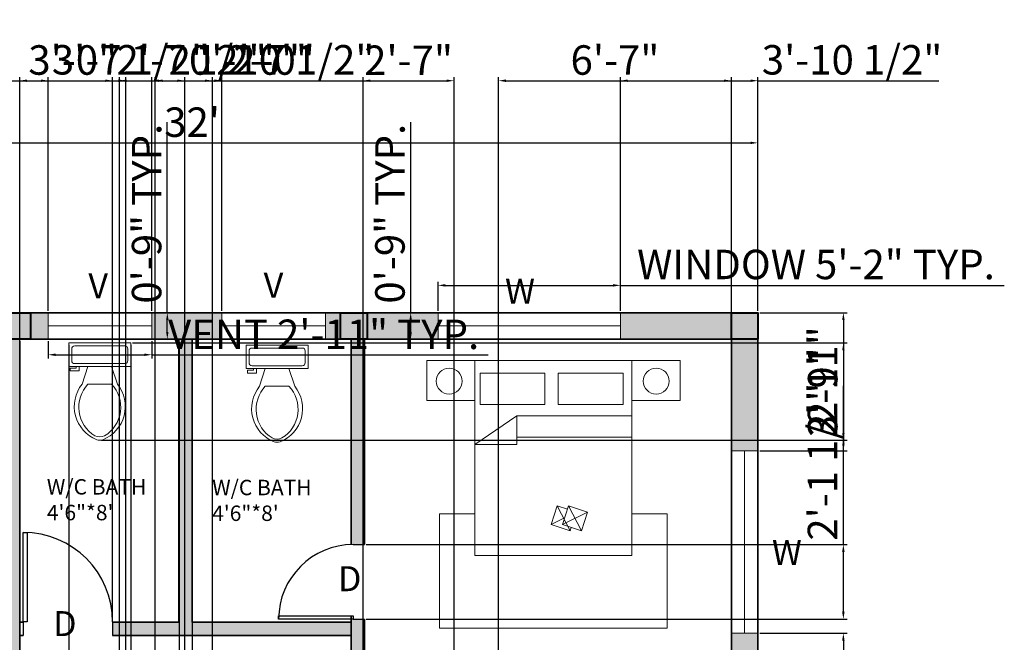
# Model space of a CAD drawing. Units: inches. Extents: x 1801 to 2333, y 2020 to 2714.
# Tile 4 of 4: x 1999 to 2333, y 2502 to 2714. Entities that reach past the tile are written whole.
import ezdxf

# ---------------------------------------------------------------- set-up
doc = ezdxf.new("R2010")
doc.units = ezdxf.units.IN
for name, color, linetype, lineweight in [('A-ANNO-DIMS', 2, 'Continuous', 18), ('A-ANNO-TEXT', 200, 'Continuous', 18), ('A-AREA-IDEN', 200, 'Continuous', 25), ('A-COLS', 7, 'Continuous', 40), ('A-COLS-PATT', 250, 'Continuous', 13), ('A-DOOR', 4, 'Continuous', 25), ('A-FLOR-FIXT', 9, 'Continuous', 18), ('A-FURN', 8, 'Continuous', 18), ('A-WALL-PATT', 252, 'Continuous', 13), ('WALL', 150, 'Continuous', 35), ('WINDOW', 130, 'Continuous', 18)]:
    doc.layers.add(name, color=color, linetype=linetype, lineweight=lineweight)
doc.styles.get("Standard").update_dxf_attribs({"font": 'arial.ttf'})
doc.dimstyles.new('ISO-25', dxfattribs={"dimtxt": 10, "dimasz": 2.5, "dimexe": 1.25, "dimexo": 0.625, "dimtad": 1, "dimdec": 0, "dimlunit": 4, "dimtxsty": 'Standard', "dimcen": 2.5, "dimadec": 0, "dimazin": 0, "dimtfac": 1, "dimtdec": 0, "dimtmove": 0, "dimatfit": 3, "dimfxl": 1, "dimarcsym": 0})

# ---------------------------------------------------------------- blocks, each defined once
blk = doc.blocks.new('*U2')
for p, q in [((0, 0), (0, -6)), ((40, 0), (40, -6))]:
    blk.add_line(p, q)
blk.add_lwpolyline([(0, 0), (0, 40), (1.75, 40), (1.75, 0)], close=True)
blk.add_arc((0, 0), 40, 0, 90)
blk = doc.blocks.new('*U4')
for p, q in [((9.5, -6), (9.5, -2)), ((-10, -8.5), (-8, -8.5)), ((-10, -9.5), (-10, -8.5)), ((-7, -9.5), (-10, -9.5)), ((-8, -8.5), (-8, -8)), ((-7, -8), (-7, -9.5)), ((-4, -8), (-6, -14)), ((4, -8), (6, -14)), ((4, -14), (-4, -14))]:
    blk.add_line(p, q)
blk.add_lwpolyline([(10.5, -8), (10.5, 0), (-10.5, 0), (-10.5, -8)], close=True)
for points in [[(-9.5, -2), (-9.5, -6)], [(8.5, -1), (-8.5, -1)], [(-8.5, -7), (8.5, -7)]]:
    blk.add_lwpolyline(points)
for centre, radius, start, end in [((-8.62, -1.88), 0.884, 81.8699, 188.1301), ((8.62, -1.88), 0.884, 351.8699, 98.1301), ((-8.62, -6.12), 0.884, 171.8699, 278.1301), ((8.62, -6.12), 0.884, 261.8699, 8.1301), ((3.52, -21.58), 12.17, 141.4691, 247.9714), ((4.2, -21.82), 11.33, 136.3677, 238.9468), ((-3.52, -21.58), 12.17, 292.0284, 38.5307), ((-4.2, -21.82), 11.33, 301.053, 43.6321), ((0, -27.88), 4, 245.7318, 294.2682), ((0, -29), 4, 254.8605, 285.1395)]:
    blk.add_arc(centre, radius, start, end)
blk = doc.blocks.new('*D7')
at = {"layer": 'A-ANNO-DIMS', "color": 0, "lineweight": -2, "transparency": 16777216}
for p, q in [((1865.69, 2614.97), (1865.69, 2673.24)), ((2249.69, 2614.97), (2249.69, 2673.24)), ((1868.19, 2671.99), (2247.19, 2671.99))]:
    blk.add_line(p, q, dxfattribs=at)
at = {"layer": 'A-ANNO-DIMS', "color": 0, "transparency": 16777216}
for points in [[(1868.19, 2672.4), (1868.19, 2671.57), (1865.69, 2671.99)], [(2247.19, 2672.4), (2247.19, 2671.57), (2249.69, 2671.99)]]:
    blk.add_solid(points, dxfattribs=at)
at = {"layer": 'Defpoints', "color": 0, "transparency": 16777216}
for p in [(2249.69, 2671.99), (1865.69, 2614.35), (2249.69, 2614.35)]:
    blk.add_point(p, dxfattribs=at)
at = {"layer": 'A-ANNO-DIMS', "color": 0, "transparency": 16777216, "insert": (2057.69, 2677.72), "char_height": 10, "attachment_point": 5}
blk.add_mtext("32'", dxfattribs=at)
blk = doc.blocks.new('BED-DOUBLE-WITH-NIGHTSTANDS')
for p, q in [((30.54, 72.05), (16.34, 62.37)), ((69.61, 72.05), (30.54, 72.05)), ((30.54, 62.37), (30.54, 72.05)), ((30.54, 64.89), (69.61, 64.89)), ((16.34, 62.37), (30.54, 62.37)), ((44.26, 41.5), (48.62, 33.08)), ((48.1, 41.5), (52.46, 33.08)), ((16.34, 38.79), (4.34, 38.79)), ((4.34, 38.79), (4.34, 0)), ((42.19, 35.19), (46.77, 37.46)), ((46.03, 35.19), (54.53, 39.39)), ((69.61, 38.79), (81.61, 38.79)), ((81.61, 38.79), (81.61, 0)), ((4.34, 0), (81.61, 0))]:
    blk.add_line(p, q)
for points in [[(0, 90.88), (16.34, 90.88), (16.34, 77.31), (0, 77.31)], [(16.34, 90.88), (69.61, 90.88), (69.61, 24.72), (16.34, 24.72)], [(69.61, 90.88), (85.96, 90.88), (85.96, 77.31), (69.61, 77.31)], [(18.06, 86.51), (40.1, 86.51), (40.1, 75.9), (18.06, 75.9)], [(44.61, 86.51), (66.65, 86.51), (66.65, 75.9), (44.61, 75.9)], [(46.03, 35.19), (48.1, 41.5), (54.53, 39.39), (52.46, 33.08)]]:
    blk.add_lwpolyline(points, close=True)
blk.add_lwpolyline([(48.99, 34.22), (48.62, 33.08), (42.19, 35.19), (44.26, 41.5), (47.73, 40.36)])
for centre in [(7.61, 83.86), (77.85, 83.86)]:
    blk.add_circle(centre, 4.4)
blk = doc.blocks.new('WIN-STANDARD')
blk.add_line((0, 4.5), (61.87, 4.5))
blk.add_lwpolyline([(0, 9), (61.87, 9), (61.87, 0), (0, 0)], close=True)
blk = doc.blocks.new('VENT-BATH')
blk.add_line((0, 4.5), (35.14, 4.5))
blk.add_lwpolyline([(0, 9), (35.14, 9), (35.14, 0), (0, 0)], close=True)
blk = doc.blocks.new('COLUMN-9X9')
blk.add_lwpolyline([(0, 9), (9, 9), (9, 0), (0, 0)], close=True)
blk = doc.blocks.new('*D18')
at = {"layer": 'A-ANNO-DIMS', "color": 0, "lineweight": -2, "transparency": 16777216}
for p, q in [((2141.14, 2614.97), (2141.14, 2624.88)), ((2143.64, 2623.63), (2200.51, 2623.63)), ((2203.01, 2614.97), (2203.01, 2624.88)), ((2203.01, 2623.63), (2333.3, 2623.63))]:
    blk.add_line(p, q, dxfattribs=at)
at = {"layer": 'A-ANNO-DIMS', "color": 0, "transparency": 16777216}
for points in [[(2143.64, 2624.05), (2143.64, 2623.21), (2141.14, 2623.63)], [(2200.51, 2624.05), (2200.51, 2623.21), (2203.01, 2623.63)]]:
    blk.add_solid(points, dxfattribs=at)
at = {"layer": 'Defpoints', "color": 0, "transparency": 16777216}
for p in [(2203.01, 2623.63), (2141.14, 2614.35), (2203.01, 2614.35)]:
    blk.add_point(p, dxfattribs=at)
at = {"layer": 'A-ANNO-DIMS', "color": 0, "transparency": 16777216, "insert": (2269.4, 2629.43), "char_height": 10, "attachment_point": 5}
blk.add_mtext('WINDOW 5\'-2" TYP.', dxfattribs=at)
blk = doc.blocks.new('*D19')
at = {"layer": 'A-ANNO-DIMS', "color": 0, "lineweight": -2, "transparency": 16777216}
for p, q in [((2131.86, 2614.35), (2131.86, 2679.05)), ((2140.51, 2614.35), (2130.61, 2614.35)), ((2131.86, 2607.85), (2131.86, 2611.85)), ((2140.51, 2605.35), (2130.61, 2605.35))]:
    blk.add_line(p, q, dxfattribs=at)
at = {"layer": 'A-ANNO-DIMS', "color": 0, "transparency": 16777216}
for points in [[(2131.44, 2611.85), (2132.27, 2611.85), (2131.86, 2614.35)], [(2131.44, 2607.85), (2132.27, 2607.85), (2131.86, 2605.35)]]:
    blk.add_solid(points, dxfattribs=at)
at = {"layer": 'Defpoints', "color": 0, "transparency": 16777216}
for p in [(2131.86, 2614.35), (2141.14, 2614.35), (2141.14, 2605.35)]:
    blk.add_point(p, dxfattribs=at)
at = {"layer": 'A-ANNO-DIMS', "color": 0, "transparency": 16777216, "insert": (2126.13, 2647.95), "char_height": 10, "attachment_point": 5, "rotation": 90}
blk.add_mtext('0\'-9" TYP.', dxfattribs=at)
blk = doc.blocks.new('*D20')
at = {"layer": 'A-ANNO-DIMS', "color": 0, "lineweight": -2, "transparency": 16777216}
for p, q in [((2008.88, 2604.72), (2008.88, 2598.83)), ((2044.01, 2604.72), (2044.01, 2598.83)), ((2011.38, 2600.08), (2041.51, 2600.08)), ((2044.01, 2600.08), (2158.14, 2600.08))]:
    blk.add_line(p, q, dxfattribs=at)
at = {"layer": 'A-ANNO-DIMS', "color": 0, "transparency": 16777216}
for points in [[(2011.38, 2600.5), (2011.38, 2599.66), (2008.88, 2600.08)], [(2041.51, 2600.5), (2041.51, 2599.66), (2044.01, 2600.08)]]:
    blk.add_solid(points, dxfattribs=at)
at = {"layer": 'Defpoints', "color": 0, "transparency": 16777216}
for p in [(2008.88, 2605.35), (2044.01, 2605.35), (2044.01, 2600.08)]:
    blk.add_point(p, dxfattribs=at)
at = {"layer": 'A-ANNO-DIMS', "color": 0, "transparency": 16777216, "insert": (2102.33, 2605.73), "char_height": 10, "attachment_point": 5}
blk.add_mtext('VENT 2\'-11" TYP.', dxfattribs=at)
blk = doc.blocks.new('*D21')
at = {"layer": 'A-ANNO-DIMS', "color": 0, "lineweight": -2, "transparency": 16777216}
for p, q in [((2049.28, 2614.35), (2049.28, 2679.05)), ((2044.64, 2614.35), (2050.53, 2614.35)), ((2049.28, 2607.85), (2049.28, 2611.85)), ((2044.64, 2605.35), (2050.53, 2605.35))]:
    blk.add_line(p, q, dxfattribs=at)
at = {"layer": 'A-ANNO-DIMS', "color": 0, "transparency": 16777216}
for points in [[(2048.86, 2611.85), (2049.7, 2611.85), (2049.28, 2614.35)], [(2048.86, 2607.85), (2049.7, 2607.85), (2049.28, 2605.35)]]:
    blk.add_solid(points, dxfattribs=at)
at = {"layer": 'Defpoints', "color": 0, "transparency": 16777216}
for p in [(2044.01, 2614.35), (2049.28, 2614.35), (2044.01, 2605.35)]:
    blk.add_point(p, dxfattribs=at)
at = {"layer": 'A-ANNO-DIMS', "color": 0, "transparency": 16777216, "insert": (2043.55, 2647.95), "char_height": 10, "attachment_point": 5, "rotation": 90}
blk.add_mtext('0\'-9" TYP.', dxfattribs=at)
blk = doc.blocks.new('*D31')
at = {"layer": 'A-ANNO-DIMS', "color": 0, "lineweight": -2, "transparency": 16777216}
for p, q in [((1965.46, 2614.97), (1965.46, 2694.33)), ((1967.96, 2693.08), (2006.38, 2693.08)), ((2008.88, 2614.97), (2008.88, 2694.33)), ((2008.88, 2693.08), (2062.5, 2693.08))]:
    blk.add_line(p, q, dxfattribs=at)
at = {"layer": 'A-ANNO-DIMS', "color": 0, "transparency": 16777216}
for points in [[(1967.96, 2693.5), (1967.96, 2692.66), (1965.46, 2693.08)], [(2006.38, 2693.5), (2006.38, 2692.66), (2008.88, 2693.08)]]:
    blk.add_solid(points, dxfattribs=at)
at = {"layer": 'Defpoints', "color": 0, "transparency": 16777216}
for p in [(2008.88, 2693.08), (1965.46, 2614.35), (2008.88, 2614.35)]:
    blk.add_point(p, dxfattribs=at)
at = {"layer": 'A-ANNO-DIMS', "color": 0, "transparency": 16777216, "insert": (2036.94, 2698.88), "char_height": 10, "attachment_point": 5}
blk.add_mtext('3\'-7 1/2"', dxfattribs=at)
blk = doc.blocks.new('*D32')
at = {"layer": 'A-ANNO-DIMS', "color": 0, "lineweight": -2, "transparency": 16777216}
for p, q in [((2044.01, 2614.97), (2044.01, 2694.33)), ((2046.51, 2693.08), (2065.29, 2693.08)), ((2067.79, 2614.97), (2067.79, 2694.33)), ((2067.79, 2693.08), (2098.29, 2693.08))]:
    blk.add_line(p, q, dxfattribs=at)
at = {"layer": 'A-ANNO-DIMS', "color": 0, "transparency": 16777216}
for points in [[(2046.51, 2693.5), (2046.51, 2692.66), (2044.01, 2693.08)], [(2065.29, 2693.5), (2065.29, 2692.66), (2067.79, 2693.08)]]:
    blk.add_solid(points, dxfattribs=at)
at = {"layer": 'Defpoints', "color": 0, "transparency": 16777216}
for p in [(2067.79, 2693.08), (2044.01, 2614.35), (2067.79, 2614.35)]:
    blk.add_point(p, dxfattribs=at)
at = {"layer": 'A-ANNO-DIMS', "color": 0, "transparency": 16777216, "insert": (2084.29, 2698.81), "char_height": 10, "attachment_point": 5}
blk.add_mtext('2\'-0"', dxfattribs=at)
blk = doc.blocks.new('*D33')
at = {"layer": 'A-ANNO-DIMS', "color": 0, "lineweight": -2, "transparency": 16777216}
for p, q in [((2203.01, 2614.97), (2203.01, 2694.33)), ((2205.51, 2693.08), (2247.19, 2693.08)), ((2249.69, 2614.97), (2249.69, 2694.33)), ((2249.69, 2693.08), (2311.09, 2693.08))]:
    blk.add_line(p, q, dxfattribs=at)
at = {"layer": 'A-ANNO-DIMS', "color": 0, "transparency": 16777216}
for points in [[(2205.51, 2693.5), (2205.51, 2692.66), (2203.01, 2693.08)], [(2247.19, 2693.5), (2247.19, 2692.66), (2249.69, 2693.08)]]:
    blk.add_solid(points, dxfattribs=at)
at = {"layer": 'Defpoints', "color": 0, "transparency": 16777216}
for p in [(2249.69, 2693.08), (2203.01, 2614.35), (2249.69, 2614.35)]:
    blk.add_point(p, dxfattribs=at)
at = {"layer": 'A-ANNO-DIMS', "color": 0, "transparency": 16777216, "insert": (2281.64, 2698.88), "char_height": 10, "attachment_point": 5}
blk.add_mtext('3\'-10 1/2"', dxfattribs=at)
blk = doc.blocks.new('*D37')
at = {"layer": 'A-ANNO-DIMS', "color": 0, "lineweight": -2, "transparency": 16777216}
for p, q in [((2250.31, 2614.35), (2279.94, 2614.35)), ((2278.69, 2611.85), (2278.69, 2569.96)), ((2250.31, 2567.46), (2279.94, 2567.46))]:
    blk.add_line(p, q, dxfattribs=at)
at = {"layer": 'A-ANNO-DIMS', "color": 0, "transparency": 16777216}
for points in [[(2278.27, 2611.85), (2279.11, 2611.85), (2278.69, 2614.35)], [(2278.27, 2569.96), (2279.11, 2569.96), (2278.69, 2567.46)]]:
    blk.add_solid(points, dxfattribs=at)
at = {"layer": 'Defpoints', "color": 0, "transparency": 16777216}
for p in [(2249.69, 2614.35), (2249.69, 2567.46), (2278.69, 2567.46)]:
    blk.add_point(p, dxfattribs=at)
at = {"layer": 'A-ANNO-DIMS', "color": 0, "transparency": 16777216, "insert": (2272.95, 2590.91), "char_height": 10, "attachment_point": 5, "rotation": 90}
blk.add_mtext('3\'-11"', dxfattribs=at)
blk = doc.blocks.new('*D38')
at = {"layer": 'A-ANNO-DIMS', "color": 0, "lineweight": -2, "transparency": 16777216}
for p, q in [((2250.31, 2505.59), (2279.94, 2505.59)), ((2278.69, 2503.09), (2278.69, 2426.51)), ((2250.31, 2424.01), (2279.94, 2424.01))]:
    blk.add_line(p, q, dxfattribs=at)
at = {"layer": 'A-ANNO-DIMS', "color": 0, "transparency": 16777216}
for points in [[(2278.27, 2503.09), (2279.11, 2503.09), (2278.69, 2505.59)], [(2278.27, 2426.51), (2279.11, 2426.51), (2278.69, 2424.01)]]:
    blk.add_solid(points, dxfattribs=at)
at = {"layer": 'Defpoints', "color": 0, "transparency": 16777216}
for p in [(2249.69, 2505.59), (2249.69, 2424.01), (2278.69, 2424.01)]:
    blk.add_point(p, dxfattribs=at)
at = {"layer": 'A-ANNO-DIMS', "color": 0, "transparency": 16777216, "insert": (2272.89, 2464.8), "char_height": 10, "attachment_point": 5, "rotation": 90}
blk.add_mtext('6\'-9 1/2"', dxfattribs=at)
blk = doc.blocks.new('*D44')
at = {"layer": 'A-ANNO-DIMS', "color": 0, "lineweight": -2, "transparency": 16777216}
for p, q in [((1999.19, 2239.97), (1999.19, 2694.33)), ((2001.69, 2693.08), (2032.69, 2693.08)), ((2035.19, 2239.97), (2035.19, 2694.33))]:
    blk.add_line(p, q, dxfattribs=at)
at = {"layer": 'A-ANNO-DIMS', "color": 0, "transparency": 16777216}
for points in [[(2001.69, 2693.5), (2001.69, 2692.66), (1999.19, 2693.08)], [(2032.69, 2693.5), (2032.69, 2692.66), (2035.19, 2693.08)]]:
    blk.add_solid(points, dxfattribs=at)
at = {"layer": 'Defpoints', "color": 0, "transparency": 16777216}
for p in [(2035.19, 2693.08), (1999.19, 2239.35), (2035.19, 2239.35)]:
    blk.add_point(p, dxfattribs=at)
at = {"layer": 'A-ANNO-DIMS', "color": 0, "transparency": 16777216, "insert": (2017.19, 2698.81), "char_height": 10, "attachment_point": 5}
blk.add_mtext('3\'-0"', dxfattribs=at)
blk = doc.blocks.new('*D45')
at = {"layer": 'A-ANNO-DIMS', "color": 0, "lineweight": -2, "transparency": 16777216}
for p, q in [((2045.19, 2143.97), (2045.19, 2694.33)), ((2047.69, 2693.08), (2052.69, 2693.08)), ((2055.19, 2143.97), (2055.19, 2694.33)), ((2055.19, 2693.08), (2093.29, 2693.08))]:
    blk.add_line(p, q, dxfattribs=at)
at = {"layer": 'A-ANNO-DIMS', "color": 0, "transparency": 16777216}
for points in [[(2047.69, 2693.5), (2047.69, 2692.66), (2045.19, 2693.08)], [(2052.69, 2693.5), (2052.69, 2692.66), (2055.19, 2693.08)]]:
    blk.add_solid(points, dxfattribs=at)
at = {"layer": 'Defpoints', "color": 0, "transparency": 16777216}
for p in [(2055.19, 2693.08), (2045.19, 2143.35), (2055.19, 2143.35)]:
    blk.add_point(p, dxfattribs=at)
at = {"layer": 'A-ANNO-DIMS', "color": 0, "transparency": 16777216, "insert": (2075.49, 2698.81), "char_height": 10, "attachment_point": 5}
blk.add_mtext('0\'-10"', dxfattribs=at)
blk = doc.blocks.new('*D47')
at = {"layer": 'A-ANNO-DIMS', "color": 0, "lineweight": -2, "transparency": 16777216}
for p, q in [((2053.36, 2604.46), (2053.36, 2104.1)), ((2057.69, 2604.72), (2057.69, 2104.1)), ((2050.86, 2105.35), (2048.36, 2105.35)), ((2053.36, 2105.35), (2057.69, 2105.35)), ((2060.19, 2105.35), (2113.82, 2105.35))]:
    blk.add_line(p, q, dxfattribs=at)
at = {"layer": 'A-ANNO-DIMS', "color": 0, "transparency": 16777216}
for points in [[(2050.86, 2105.76), (2050.86, 2104.93), (2053.36, 2105.35)], [(2060.19, 2105.76), (2060.19, 2104.93), (2057.69, 2105.35)]]:
    blk.add_solid(points, dxfattribs=at)
at = {"layer": 'Defpoints', "color": 0, "transparency": 16777216}
for p in [(2053.36, 2605.08), (2057.69, 2605.35), (2057.69, 2105.35)]:
    blk.add_point(p, dxfattribs=at)
at = {"layer": 'A-ANNO-DIMS', "color": 0, "transparency": 16777216, "insert": (2088.26, 2111.14), "char_height": 10, "attachment_point": 5}
blk.add_mtext('0\'-4 1/2"', dxfattribs=at)
blk = doc.blocks.new('*D49')
at = {"layer": 'A-ANNO-DIMS', "color": 0, "lineweight": -2, "transparency": 16777216}
for p, q in [((1999.19, 2509.97), (1999.19, 2694.33)), ((2001.69, 2693.08), (2028.22, 2693.08)), ((2030.72, 2509.97), (2030.72, 2694.33)), ((2030.72, 2693.08), (2084.53, 2693.08))]:
    blk.add_line(p, q, dxfattribs=at)
at = {"layer": 'A-ANNO-DIMS', "color": 0, "transparency": 16777216}
for points in [[(2001.69, 2693.5), (2001.69, 2692.66), (1999.19, 2693.08)], [(2028.22, 2693.5), (2028.22, 2692.66), (2030.72, 2693.08)]]:
    blk.add_solid(points, dxfattribs=at)
at = {"layer": 'Defpoints', "color": 0, "transparency": 16777216}
for p in [(2030.72, 2693.08), (1999.19, 2509.35), (2030.72, 2509.35)]:
    blk.add_point(p, dxfattribs=at)
at = {"layer": 'A-ANNO-DIMS', "color": 0, "transparency": 16777216, "insert": (2058.88, 2698.88), "char_height": 10, "attachment_point": 5}
blk.add_mtext('2\'-7 1/2"', dxfattribs=at)
blk = doc.blocks.new('*D50')
at = {"layer": 'A-ANNO-DIMS', "color": 0, "lineweight": -2, "transparency": 16777216}
for p, q in [((2278.69, 2535.68), (2278.69, 2589.49)), ((2116.81, 2535.68), (2279.94, 2535.68)), ((2278.69, 2512.85), (2278.69, 2533.18)), ((2116.81, 2510.35), (2279.94, 2510.35))]:
    blk.add_line(p, q, dxfattribs=at)
at = {"layer": 'A-ANNO-DIMS', "color": 0, "transparency": 16777216}
for points in [[(2278.27, 2533.18), (2279.11, 2533.18), (2278.69, 2535.68)], [(2278.27, 2512.85), (2279.11, 2512.85), (2278.69, 2510.35)]]:
    blk.add_solid(points, dxfattribs=at)
at = {"layer": 'Defpoints', "color": 0, "transparency": 16777216}
for p in [(2116.19, 2535.68), (2278.69, 2535.68), (2116.19, 2510.35)]:
    blk.add_point(p, dxfattribs=at)
at = {"layer": 'A-ANNO-DIMS', "color": 0, "transparency": 16777216, "insert": (2272.89, 2563.83), "char_height": 10, "attachment_point": 5, "rotation": 90}
blk.add_mtext('2\'-1 1/2"', dxfattribs=at)
blk = doc.blocks.new('*D51')
at = {"layer": 'A-ANNO-DIMS', "color": 0, "lineweight": -2, "transparency": 16777216}
for p, q in [((2033.02, 2423.43), (2033.02, 2694.33)), ((2035.52, 2693.08), (2062.07, 2693.08)), ((2064.57, 2423.43), (2064.57, 2694.33)), ((2064.57, 2693.08), (2118.37, 2693.08))]:
    blk.add_line(p, q, dxfattribs=at)
at = {"layer": 'A-ANNO-DIMS', "color": 0, "transparency": 16777216}
for points in [[(2035.52, 2693.5), (2035.52, 2692.66), (2033.02, 2693.08)], [(2062.07, 2693.5), (2062.07, 2692.66), (2064.57, 2693.08)]]:
    blk.add_solid(points, dxfattribs=at)
at = {"layer": 'Defpoints', "color": 0, "transparency": 16777216}
for p in [(2064.57, 2693.08), (2033.02, 2422.8), (2064.57, 2422.8)]:
    blk.add_point(p, dxfattribs=at)
at = {"layer": 'A-ANNO-DIMS', "color": 0, "transparency": 16777216, "insert": (2092.72, 2698.88), "char_height": 10, "attachment_point": 5}
blk.add_mtext('2\'-7 1/2"', dxfattribs=at)
blk = doc.blocks.new('*D53')
at = {"layer": 'A-ANNO-DIMS', "color": 0, "lineweight": -2, "transparency": 16777216}
for p, q in [((2115.69, 2274.54), (2115.69, 2694.33)), ((2118.19, 2693.08), (2144.09, 2693.08)), ((2146.59, 2274.54), (2146.59, 2694.33))]:
    blk.add_line(p, q, dxfattribs=at)
at = {"layer": 'A-ANNO-DIMS', "color": 0, "transparency": 16777216}
for points in [[(2118.19, 2693.5), (2118.19, 2692.66), (2115.69, 2693.08)], [(2144.09, 2693.5), (2144.09, 2692.66), (2146.59, 2693.08)]]:
    blk.add_solid(points, dxfattribs=at)
at = {"layer": 'Defpoints', "color": 0, "transparency": 16777216}
for p in [(2146.59, 2693.08), (2115.69, 2273.91), (2146.59, 2273.91)]:
    blk.add_point(p, dxfattribs=at)
at = {"layer": 'A-ANNO-DIMS', "color": 0, "transparency": 16777216, "insert": (2131.14, 2698.73), "char_height": 10, "attachment_point": 5}
blk.add_mtext('2\'-7"', dxfattribs=at)
blk = doc.blocks.new('*D54')
at = {"layer": 'A-ANNO-DIMS', "color": 0, "lineweight": -2, "transparency": 16777216}
for p, q in [((2161.67, 2353.47), (2161.67, 2694.33)), ((2164.17, 2693.08), (2238.19, 2693.08)), ((2240.69, 2353.47), (2240.69, 2694.33))]:
    blk.add_line(p, q, dxfattribs=at)
at = {"layer": 'A-ANNO-DIMS', "color": 0, "transparency": 16777216}
for points in [[(2164.17, 2693.5), (2164.17, 2692.66), (2161.67, 2693.08)], [(2238.19, 2693.5), (2238.19, 2692.66), (2240.69, 2693.08)]]:
    blk.add_solid(points, dxfattribs=at)
at = {"layer": 'Defpoints', "color": 0, "transparency": 16777216}
for p in [(2240.69, 2693.08), (2161.67, 2352.85), (2240.69, 2352.85)]:
    blk.add_point(p, dxfattribs=at)
at = {"layer": 'A-ANNO-DIMS', "color": 0, "transparency": 16777216, "insert": (2201.18, 2698.81), "char_height": 10, "attachment_point": 5}
blk.add_mtext('6\'-7"', dxfattribs=at)
blk = doc.blocks.new('*D55')
at = {"layer": 'A-ANNO-DIMS', "color": 0, "lineweight": -2, "transparency": 16777216}
for p, q in [((1999.19, 2604.72), (1999.19, 2104.1)), ((2015.86, 2603.46), (2015.86, 2104.1)), ((2001.69, 2105.35), (2013.36, 2105.35)), ((2015.86, 2105.35), (2068.55, 2105.35))]:
    blk.add_line(p, q, dxfattribs=at)
at = {"layer": 'A-ANNO-DIMS', "color": 0, "transparency": 16777216}
for points in [[(2001.69, 2105.76), (2001.69, 2104.93), (1999.19, 2105.35)], [(2013.36, 2105.76), (2013.36, 2104.93), (2015.86, 2105.35)]]:
    blk.add_solid(points, dxfattribs=at)
at = {"layer": 'Defpoints', "color": 0, "transparency": 16777216}
for p in [(1999.19, 2605.35), (2015.86, 2604.08), (2015.86, 2105.35)]:
    blk.add_point(p, dxfattribs=at)
at = {"layer": 'A-ANNO-DIMS', "color": 0, "transparency": 16777216, "insert": (2043.46, 2111.14), "char_height": 10, "attachment_point": 5}
blk.add_mtext('1\'-4 1/2"', dxfattribs=at)
blk = doc.blocks.new('*D56')
at = {"layer": 'A-ANNO-DIMS', "color": 0, "lineweight": -2, "transparency": 16777216}
for p, q in [((2015.86, 2603.46), (2015.86, 2104.1)), ((2036.86, 2603.46), (2036.86, 2104.1)), ((2018.36, 2105.35), (2034.36, 2105.35)), ((2036.86, 2105.35), (2066.25, 2105.35))]:
    blk.add_line(p, q, dxfattribs=at)
at = {"layer": 'A-ANNO-DIMS', "color": 0, "transparency": 16777216}
for points in [[(2018.36, 2105.76), (2018.36, 2104.93), (2015.86, 2105.35)], [(2034.36, 2105.76), (2034.36, 2104.93), (2036.86, 2105.35)]]:
    blk.add_solid(points, dxfattribs=at)
at = {"layer": 'Defpoints', "color": 0, "transparency": 16777216}
for p in [(2015.86, 2604.08), (2036.86, 2604.08), (2036.86, 2105.35)]:
    blk.add_point(p, dxfattribs=at)
at = {"layer": 'A-ANNO-DIMS', "color": 0, "transparency": 16777216, "insert": (2052.81, 2111.08), "char_height": 10, "attachment_point": 5}
blk.add_mtext('1\'-9"', dxfattribs=at)
blk = doc.blocks.new('*D57')
at = {"layer": 'A-ANNO-DIMS', "color": 0, "lineweight": -2, "transparency": 16777216}
for p, q in [((2037.49, 2604.08), (2279.94, 2604.08)), ((2278.69, 2601.58), (2278.69, 2573.58)), ((2026.99, 2571.08), (2279.94, 2571.08))]:
    blk.add_line(p, q, dxfattribs=at)
at = {"layer": 'A-ANNO-DIMS', "color": 0, "transparency": 16777216}
for points in [[(2278.27, 2601.58), (2279.11, 2601.58), (2278.69, 2604.08)], [(2278.27, 2573.58), (2279.11, 2573.58), (2278.69, 2571.08)]]:
    blk.add_solid(points, dxfattribs=at)
at = {"layer": 'Defpoints', "color": 0, "transparency": 16777216}
for p in [(2036.86, 2604.08), (2026.36, 2571.08), (2278.69, 2571.08)]:
    blk.add_point(p, dxfattribs=at)
at = {"layer": 'A-ANNO-DIMS', "color": 0, "transparency": 16777216, "insert": (2272.96, 2587.58), "char_height": 10, "attachment_point": 5, "rotation": 90}
blk.add_mtext('2\'-9"', dxfattribs=at)

msp = doc.modelspace()

# ---------------------------------------------------------------- hatches: boundary and pattern name
at = {"layer": 'A-COLS-PATT'}
h = msp.add_hatch(color=256, dxfattribs=at)
h.dxf.hatch_style = 1
h.paths.add_polyline_path([(1874.69, 2614.35), (1865.69, 2614.35), (1865.69, 2605.35), (1874.69, 2605.35)])
h.paths.add_polyline_path([(2002.83, 2614.35), (1993.83, 2614.35), (1993.83, 2605.35), (2002.83, 2605.35)])
h.paths.add_polyline_path([(2117.06, 2614.35), (2108.06, 2614.35), (2108.06, 2605.35), (2117.06, 2605.35)])
h.paths.add_polyline_path([(2249.69, 2614.35), (2240.69, 2614.35), (2240.69, 2605.35), (2249.69, 2605.35)])
h.paths.add_polyline_path([(1874.69, 2452.27), (1865.69, 2452.27), (1865.69, 2443.27), (1874.69, 2443.27)])
h.paths.add_polyline_path([(1999.19, 2449.12), (1990.19, 2449.12), (1990.19, 2444.85), (1999.19, 2444.85)])
h.paths.add_polyline_path([(1999.19, 2444.85), (1990.19, 2444.85), (1990.19, 2440.12), (1999.19, 2440.12)])
h.paths.add_polyline_path([(2120.9, 2449.35), (2116.19, 2449.35), (2116.19, 2453.56), (2111.9, 2453.56), (2111.9, 2444.85), (2120.9, 2444.85)])
h.paths.add_polyline_path([(2120.9, 2453.56), (2116.19, 2453.56), (2116.19, 2449.35), (2120.9, 2449.35)], flags=17)
h.paths.add_polyline_path([(2249.69, 2451.04), (2240.69, 2451.04), (2240.69, 2442.04), (2249.69, 2442.04)])
h.paths.add_polyline_path([(2249.69, 2330.92), (2240.69, 2330.92), (2240.69, 2321.92), (2249.69, 2321.92)])
h.paths.add_polyline_path([(2115.69, 2329.7), (2111.19, 2329.7), (2111.19, 2324.35), (2115.69, 2324.35)])
h.paths.add_polyline_path([(2115.69, 2324.35), (2111.19, 2324.35), (2111.19, 2320.7), (2115.69, 2320.7)])
h.paths.add_polyline_path([(2111.19, 2329.7), (2106.69, 2329.7), (2106.69, 2320.7), (2111.19, 2320.7), (2111.19, 2324.35)])
h.paths.add_polyline_path([(1999.19, 2291.85), (1991.86, 2291.85), (1991.86, 2287.35), (1994.69, 2287.35), (1994.69, 2283.08), (1999.19, 2283.08)], flags=17)
h.paths.add_polyline_path([(2000.86, 2292.08), (1991.86, 2292.08), (1991.86, 2291.85), (1999.19, 2291.85), (1999.19, 2283.08), (2000.86, 2283.08)])
h.paths.add_polyline_path([(1994.69, 2287.35), (1991.86, 2287.35), (1991.86, 2283.08), (1994.69, 2283.08)], flags=16)
h.paths.add_polyline_path([(1874.69, 2143.35), (1865.69, 2143.35), (1865.69, 2134.35), (1874.69, 2134.35)])
h.paths.add_polyline_path([(1999.19, 2143.35), (1990.19, 2143.35), (1990.19, 2134.35), (1999.19, 2134.35)])
h.paths.add_polyline_path([(2118.63, 2143.35), (2109.63, 2143.35), (2109.63, 2134.35), (2118.63, 2134.35)])
h.paths.add_polyline_path([(2249.69, 2143.35), (2240.69, 2143.35), (2240.69, 2134.35), (2249.69, 2134.35)])
at = {"layer": 'A-WALL-PATT'}
h = msp.add_hatch(color=256, dxfattribs=at)
h.dxf.hatch_style = 1
h.paths.add_polyline_path([(2067.79, 2614.35), (2044.01, 2614.35), (2044.01, 2605.35), (2053.19, 2605.35), (2067.79, 2605.35)])
h.paths.add_polyline_path([(2057.69, 2605.35), (2053.19, 2605.35), (2053.19, 2509.35), (2040.35, 2509.35), (2030.72, 2509.35), (2030.72, 2504.85), (2040.35, 2504.85), (2057.69, 2504.85), (2111.69, 2504.85), (2111.69, 2509.35), (2057.69, 2509.35)])
h.paths.add_polyline_path([(1999.19, 2605.35), (1994.69, 2605.35), (1994.69, 2490.6), (1999.19, 2490.6)])
h.paths.add_polyline_path([(2116.19, 2605.35), (2111.69, 2605.35), (2111.69, 2550.35), (2111.69, 2535.67, -0.006913), (2112.39, 2535.68), (2116.19, 2535.68), (2116.19, 2551.5)])
h.paths.add_polyline_path([(2116.19, 2510.35), (2112.39, 2510.35), (2111.69, 2510.35), (2111.69, 2495.25), (2116.19, 2495.25)])
h.paths.add_polyline_path([(2115.69, 2273.91), (2111.19, 2273.91), (2111.19, 2143.35), (2115.69, 2143.35)], flags=17)
h.paths.add_polyline_path([(2118.63, 2143.35), (2118.63, 2134.35), (2159.47, 2134.35), (2159.47, 2143.35)])
h.paths.add_polyline_path([(2109.63, 2134.35), (2109.63, 2143.35), (2082.87, 2143.35), (2082.87, 2134.35)])
h.paths.add_polyline_path([(1999.19, 2143.35), (1999.19, 2134.35), (2021.01, 2134.35), (2021.01, 2143.35)])
h.paths.add_polyline_path([(1990.19, 2134.35), (1990.19, 2143.35), (1965.15, 2143.35), (1965.15, 2134.35)])
h.paths.add_polyline_path([(1903.28, 2143.35), (1874.69, 2143.35), (1874.69, 2134.35), (1903.28, 2134.35)])
h.paths.add_polyline_path([(1865.69, 2143.35), (1874.69, 2143.35), (1874.69, 2183.28), (1865.69, 2183.28)])
h.paths.add_polyline_path([(1991.86, 2287.35), (1991.86, 2291.85), (1874.69, 2291.85), (1874.69, 2287.35)])
h.paths.add_polyline_path([(1999.19, 2283.08), (1994.69, 2283.08), (1994.69, 2282.32), (1999.19, 2282.32)])
h.paths.add_polyline_path([(1865.69, 2452.27), (1874.69, 2452.27), (1874.69, 2515.15), (1865.69, 2515.15)])
h.paths.add_polyline_path([(1874.69, 2443.27), (1865.69, 2443.27), (1865.69, 2400.61), (1874.69, 2400.61)])
h.paths.add_polyline_path([(2120.9, 2449.35), (2120.9, 2444.85), (2240.69, 2444.85), (2240.69, 2449.35)])
h.paths.add_polyline_path([(2111.9, 2453.56), (2116.19, 2453.56), (2116.19, 2455.25), (2111.69, 2455.25), (2111.69, 2444.85), (2111.9, 2444.85)])
h.paths.add_polyline_path([(1874.69, 2605.35), (1865.69, 2605.35), (1865.69, 2577.02), (1874.69, 2577.02)])
h.paths.add_polyline_path([(1874.69, 2614.35), (1874.69, 2605.35), (1903.59, 2605.35), (1903.59, 2614.35)])
h = msp.add_hatch(color=256, dxfattribs=at)
h.dxf.hatch_style = 1
h.paths.add_polyline_path([(2118.63, 2143.35), (2118.63, 2134.35), (2159.47, 2134.35), (2159.47, 2143.35)])
h.paths.add_polyline_path([(2109.63, 2134.35), (2109.63, 2143.35), (2082.87, 2143.35), (2082.87, 2134.35)])
h.paths.add_polyline_path([(1999.19, 2143.35), (1999.19, 2134.35), (2021.01, 2134.35), (2021.01, 2143.35)])
h.paths.add_polyline_path([(1990.19, 2134.35), (1990.19, 2143.35), (1965.15, 2143.35), (1965.15, 2134.35)])
h.paths.add_polyline_path([(1874.69, 2143.35), (1874.69, 2134.35), (1903.28, 2134.35), (1903.28, 2143.35)])
h.paths.add_polyline_path([(1865.69, 2143.35), (1874.69, 2143.35), (1874.69, 2183.28), (1865.69, 2183.28)])
h.paths.add_polyline_path([(1874.69, 2443.27), (1865.69, 2443.27), (1865.69, 2400.61), (1874.69, 2400.61)])
h.paths.add_polyline_path([(1865.69, 2452.27), (1874.69, 2452.27), (1874.69, 2515.15), (1865.69, 2515.15)])
h.paths.add_polyline_path([(1874.69, 2577.02), (1874.69, 2605.35), (1865.69, 2605.35), (1865.69, 2577.02)])
h.paths.add_polyline_path([(1874.69, 2614.35), (1874.69, 2605.35), (1903.59, 2605.35), (1903.59, 2614.35)])
h.paths.add_polyline_path([(2240.69, 2605.35), (2240.69, 2614.35), (2203.01, 2614.35), (2203.01, 2605.35)])
h.paths.add_polyline_path([(2249.69, 2605.35), (2240.69, 2605.35), (2240.69, 2567.46), (2249.69, 2567.46)])
h = msp.add_hatch(color=256, dxfattribs=at)
h.dxf.hatch_style = 1
h.paths.add_polyline_path([(2249.69, 2505.59), (2240.69, 2505.59), (2240.69, 2451.04), (2249.69, 2451.04)])
h.paths.add_polyline_path([(2249.69, 2442.04), (2240.69, 2442.04), (2240.69, 2424.01), (2249.69, 2424.01)])
h.paths.add_polyline_path([(2249.69, 2362.14), (2240.69, 2362.14), (2240.69, 2330.92), (2249.69, 2330.92)])
h.paths.add_polyline_path([(2249.69, 2321.92), (2240.69, 2321.92), (2240.69, 2143.35), (2249.69, 2143.35)])
h.paths.add_polyline_path([(2240.69, 2143.35), (2214.05, 2143.35), (2214.05, 2134.35), (2240.69, 2134.35)])
h.paths.add_polyline_path([(1874.69, 2282.85), (1865.69, 2282.85), (1865.69, 2245.15), (1874.69, 2245.15)])
h.paths.add_polyline_path([(1874.69, 2338.74), (1865.69, 2338.74), (1865.69, 2291.85), (1874.69, 2291.85)])
h.paths.add_polyline_path([(1990.19, 2449.12), (1999.19, 2449.12), (1999.19, 2450.6), (1994.69, 2450.6), (1994.69, 2449.35), (1874.69, 2449.35), (1874.69, 2444.85), (1990.19, 2444.85)])
h.paths.add_polyline_path([(2141.14, 2614.35), (2117.06, 2614.35), (2117.06, 2605.35), (2141.14, 2605.35)])
h.paths.add_polyline_path([(2108.06, 2614.35), (2102.92, 2614.35), (2102.92, 2605.35), (2108.06, 2605.35)])
h.paths.add_polyline_path([(1993.83, 2614.35), (1965.46, 2614.35), (1965.46, 2605.35), (1993.83, 2605.35)])
h.paths.add_polyline_path([(2008.88, 2614.35), (2002.83, 2614.35), (2002.83, 2605.35), (2008.88, 2605.35)])
h.paths.add_polyline_path([(2107.38, 2466.24), (2120.18, 2466.24), (2120.18, 2483.72), (2107.38, 2483.72)], flags=9)
h.paths.add_polyline_path([(2104.14, 2515.21), (2116.94, 2515.21), (2116.94, 2532.69), (2104.14, 2532.69)], flags=9)
h.paths.add_polyline_path([(2007.5, 2499.97), (2020.3, 2499.97), (2020.3, 2517.44), (2007.5, 2517.44)], flags=9)
h.paths.add_polyline_path([(1985.91, 2461.68), (1998.7, 2461.68), (1998.7, 2479.15), (1985.91, 2479.15)], flags=9)
h.paths.add_polyline_path([(2109.98, 2348.28), (2122.78, 2348.28), (2122.78, 2365.76), (2109.98, 2365.76)], flags=9)
h.paths.add_polyline_path([(1977.13, 2255.51), (1989.93, 2255.51), (1989.93, 2272.99), (1977.13, 2272.99)], flags=9)
h.paths.add_polyline_path([(2063.1, 2540.71), (2101.48, 2540.71), (2101.48, 2560.24), (2063.1, 2560.24)], flags=9)
h.paths.add_polyline_path([(1995.81, 2316.5), (2071.83, 2316.5), (2071.83, 2348.15), (1995.81, 2348.15)], flags=9)
h.paths.add_polyline_path([(2138.31, 2394.68), (2194.97, 2394.68), (2194.97, 2426.33), (2138.31, 2426.33)], flags=9)
h.paths.add_polyline_path([(2163.82, 2472.81), (2229.7, 2472.81), (2229.7, 2504.45), (2163.82, 2504.45)], flags=9)
h.paths.add_polyline_path([(2007.01, 2540.94), (2045.38, 2540.94), (2045.38, 2560.47), (2007.01, 2560.47)], flags=9)
h.paths.add_polyline_path([(1882.98, 2452.95), (1948.86, 2452.95), (1948.86, 2484.59), (1882.98, 2484.59)], flags=9)

# ---------------------------------------------------------------- linework, layer by layer
at = {"layer": 'WALL'}
for p, q in [((1999.19, 2605.35), (2053.19, 2605.35)), ((2053.19, 2605.35), (2053.19, 2509.35)), ((2057.69, 2605.35), (2057.69, 2509.35)), ((2057.69, 2605.35), (2111.69, 2605.35)), ((2057.69, 2605.35), (2111.69, 2605.35)), ((2111.69, 2605.35), (2111.69, 2550.35)), ((2240.69, 2605.35), (2115.69, 2605.35)), ((2116.19, 2605.35), (2116.19, 2550.35)), ((2240.69, 2605.35), (2240.69, 2449.35)), ((2111.69, 2550.35), (2111.69, 2535.67)), ((2116.19, 2551.5), (2116.19, 2535.68)), ((2000.35, 2509.35), (1999.19, 2509.35)), ((2040.35, 2509.35), (2030.72, 2509.35)), ((2053.19, 2509.35), (2040.35, 2509.35)), ((2111.69, 2509.35), (2057.69, 2509.35)), ((2111.69, 2495.25), (2111.69, 2511.6)), ((2111.69, 2510.35), (2111.69, 2509.35)), ((2116.19, 2495.25), (2116.19, 2510.35)), ((2116.19, 2510.35), (2116.19, 2504.85)), ((2000.35, 2504.85), (1999.19, 2504.85)), ((2040.35, 2504.85), (2030.72, 2504.85)), ((2057.69, 2504.85), (2040.35, 2504.85)), ((2111.69, 2504.85), (2057.69, 2504.85))]:
    msp.add_line(p, q, dxfattribs=at)
for points in [[(2214.05, 2134.35), (2249.69, 2134.35), (2249.69, 2614.35), (1865.69, 2614.35), (1865.69, 2134.35), (2159.47, 2134.35)], [(2214.05, 2143.35), (2240.69, 2143.35), (2240.69, 2605.35), (1874.69, 2605.35), (1874.69, 2143.35), (2159.47, 2143.35)]]:
    msp.add_lwpolyline(points, dxfattribs=at)

# ---------------------------------------------------------------- block references
at = {"layer": 'A-COLS'}
for p in [(1993.83, 2605.35), (2108.06, 2605.35), (2240.69, 2605.35)]:
    msp.add_blockref('COLUMN-9X9', p, dxfattribs=at)
at = {"layer": 'A-DOOR', "xscale": 0.7594178637599553, "yscale": 0.7594178637599553, "zscale": 0.7594178637599553}
msp.add_blockref('*U2', (2000.35, 2509.41), dxfattribs=at)
at = {"layer": 'A-DOOR', "xscale": 0.6332703532117839, "yscale": 0.6332703532117839, "zscale": 0.6332703532117839, "rotation": 90}
msp.add_blockref('*U2', (2112.39, 2510.35), dxfattribs=at)
at = {"layer": 'A-FLOR-FIXT'}
for p in [(2026.36, 2604.08), (2086.54, 2603.37)]:
    msp.add_blockref('*U4', p, dxfattribs=at)
at = {"layer": 'A-FURN'}
msp.add_blockref('BED-DOUBLE-WITH-NIGHTSTANDS', (2137.34, 2507.27), dxfattribs=at)
at = {"layer": 'WINDOW'}
for name, p in [('VENT-BATH', (2008.88, 2605.35)), ('VENT-BATH', (2067.79, 2605.35)), ('WIN-STANDARD', (2141.14, 2605.35))]:
    msp.add_blockref(name, p, dxfattribs=at)
at = {"layer": 'WINDOW', "rotation": 269.9999999999999}
msp.add_blockref('WIN-STANDARD', (2240.69, 2567.46), dxfattribs=at)

# ---------------------------------------------------------------- texts
at = {"layer": 'A-ANNO-TEXT', "char_height": 8.48, "attachment_point": 1}
for s, insert in [('V', (2022.49, 2627.72)), ('V', (2081.98, 2627.89)), ('W', (2163.88, 2625.86)), ('W', (2254.44, 2537.24)), ('D', (2107.18, 2528.32)), ('D', (2010.54, 2513.08))]:
    msp.add_mtext_dynamic_manual_height_columns(s, width=170.2706, gutter_width=42.4, heights=[0], dxfattribs=dict(at, insert=insert))
at = {"layer": 'A-AREA-IDEN', "char_height": 5.235, "attachment_point": 1}
for insert in [(2008.41, 2557.87), (2064.5, 2557.64)]:
    msp.add_mtext_dynamic_manual_height_columns('W/C BATH\\P4\'6"*8\'', width=105.1101, gutter_width=26.18, heights=[0], dxfattribs=dict(at, insert=insert))

# ---------------------------------------------------------------- dimensions: what is measured, and where the dimension line sits
at = {"layer": 'A-ANNO-DIMS'}
for base, p1, p2, override, picture, middle in [((2008.88, 2693.08), (1965.46, 2614.35), (2008.88, 2614.35), {"dimdec": 1, "dimlfac": 1, "dimrnd": 0, "dimzin": 1, "dimdsep": 46, "dimlunit": 4, "dimfrac": 2}, '*D31', (2036.94, 2698.88)), ((2030.72, 2693.08), (1999.19, 2509.35), (2030.72, 2509.35), {"dimdec": 1, "dimlfac": 1, "dimrnd": 0, "dimzin": 1, "dimdsep": 46, "dimlunit": 4, "dimfrac": 2}, '*D49', (2058.88, 2698.88)), ((2064.5666, 2693.0804), (2033.0178, 2422.8025), (2064.5666, 2422.8025), {"dimdec": 1, "dimlfac": 1, "dimrnd": 0, "dimzin": 1, "dimdsep": 46, "dimlunit": 4, "dimfrac": 2}, '*D51', (2092.7189, 2698.8759)), ((2249.69, 2693.08), (2203.01, 2614.35), (2249.69, 2614.35), {"dimdec": 1, "dimlfac": 1, "dimrnd": 0, "dimzin": 1, "dimdsep": 46, "dimlunit": 4, "dimfrac": 2}, '*D33', (2281.64, 2698.88)), ((2035.19, 2693.08), (1999.19, 2239.35), (2035.19, 2239.35), {"dimdec": 1, "dimlfac": 1, "dimrnd": 0, "dimzin": 1, "dimdsep": 46, "dimlunit": 4, "dimfrac": 2}, '*D44', (2017.19, 2698.81)), ((2067.79, 2693.08), (2044.01, 2614.35), (2067.79, 2614.35), {"dimdec": 1, "dimlfac": 1, "dimrnd": 0, "dimzin": 1, "dimdsep": 46, "dimlunit": 4, "dimfrac": 2}, '*D32', (2084.29, 2698.81)), ((2055.19, 2693.08), (2045.19, 2143.35), (2055.19, 2143.35), {"dimdec": 1, "dimlfac": 1, "dimrnd": 0, "dimzin": 1, "dimdsep": 46, "dimlunit": 4, "dimfrac": 2}, '*D45', (2075.49, 2698.81)), ((2146.59, 2693.08), (2115.69, 2273.91), (2146.59, 2273.91), {"dimdec": 1, "dimlfac": 1, "dimrnd": 0, "dimzin": 1, "dimdsep": 46, "dimlunit": 4, "dimfrac": 2}, '*D53', (2131.14, 2698.73)), ((2240.69, 2693.08), (2161.67, 2352.85), (2240.69, 2352.85), {"dimdec": 1, "dimlfac": 1, "dimrnd": 0, "dimzin": 1, "dimdsep": 46, "dimlunit": 4, "dimfrac": 2}, '*D54', (2201.18, 2698.81)), ((2249.69, 2671.99), (1865.69, 2614.35), (2249.69, 2614.35), {"dimclrd": 0, "dimclre": 0, "dimclrt": 0}, '*D7', (2057.69, 2677.72)), ((2015.86, 2105.35), (1999.19, 2605.35), (2015.86, 2604.08), {"dimdec": 1, "dimlfac": 1, "dimrnd": 0, "dimzin": 1, "dimdsep": 46, "dimlunit": 4, "dimfrac": 2}, '*D55', (2043.46, 2111.14)), ((2036.86, 2105.35), (2015.86, 2604.08), (2036.86, 2604.08), {"dimdec": 1, "dimlfac": 1, "dimrnd": 0, "dimzin": 1, "dimdsep": 46, "dimlunit": 4, "dimfrac": 2}, '*D56', (2052.81, 2111.08)), ((2057.69, 2105.35), (2053.36, 2605.08), (2057.69, 2605.35), {"dimdec": 1, "dimlfac": 1, "dimrnd": 0, "dimzin": 1, "dimdsep": 46, "dimlunit": 4, "dimfrac": 2}, '*D47', (2088.26, 2111.14))]:
    dim = msp.add_linear_dim(base=base, p1=p1, p2=p2, dimstyle='ISO-25', override=override, dxfattribs=at)
    dim.commit()
    dim.dimension.update_dxf_attribs({"geometry": picture, "text_midpoint": middle})
for base, p1, p2, picture, middle in [((2049.28, 2614.35), (2044.01, 2605.35), (2044.01, 2614.35), '*D21', (2043.55, 2647.95)), ((2131.86, 2614.35), (2141.14, 2605.35), (2141.14, 2614.35), '*D19', (2126.13, 2647.95))]:
    dim = msp.add_linear_dim(base=base, p1=p1, p2=p2, angle=90, text='<> TYP.', dimstyle='ISO-25', override={"dimdec": 1, "dimlfac": 1, "dimrnd": 0, "dimzin": 1, "dimdsep": 46, "dimlunit": 4, "dimfrac": 2}, dxfattribs=at)
    dim.commit()
    dim.dimension.update_dxf_attribs({"geometry": picture, "text_midpoint": middle})
for base, p1, p2, text, picture, middle in [((2203.01, 2623.63), (2141.14, 2614.35), (2203.01, 2614.35), 'WINDOW <> TYP.', '*D18', (2269.4, 2629.43)), ((2044.01, 2600.08), (2008.88, 2605.35), (2044.01, 2605.35), 'VENT <> TYP.', '*D20', (2102.33, 2605.73))]:
    dim = msp.add_linear_dim(base=base, p1=p1, p2=p2, text=text, dimstyle='ISO-25', override={"dimdec": 1, "dimlfac": 1, "dimrnd": 0, "dimzin": 1, "dimdsep": 46, "dimlunit": 4, "dimfrac": 2}, dxfattribs=at)
    dim.commit()
    dim.dimension.update_dxf_attribs({"geometry": picture, "text_midpoint": middle})
for base, p1, p2, picture, middle in [((2278.69, 2567.46), (2249.69, 2614.35), (2249.69, 2567.46), '*D37', (2272.95, 2590.91)), ((2278.69, 2571.08), (2036.86, 2604.08), (2026.36, 2571.08), '*D57', (2272.96, 2587.58)), ((2278.69, 2535.68), (2116.19, 2510.35), (2116.19, 2535.68), '*D50', (2272.89, 2563.83)), ((2278.69, 2424.01), (2249.69, 2505.59), (2249.69, 2424.01), '*D38', (2272.89, 2464.8))]:
    dim = msp.add_linear_dim(base=base, p1=p1, p2=p2, angle=90, dimstyle='ISO-25', override={"dimdec": 1, "dimlfac": 1, "dimrnd": 0, "dimzin": 1, "dimdsep": 46, "dimlunit": 4, "dimfrac": 2}, dxfattribs=at)
    dim.commit()
    dim.dimension.update_dxf_attribs({"geometry": picture, "text_midpoint": middle})

doc.saveas('drawing.dxf')
